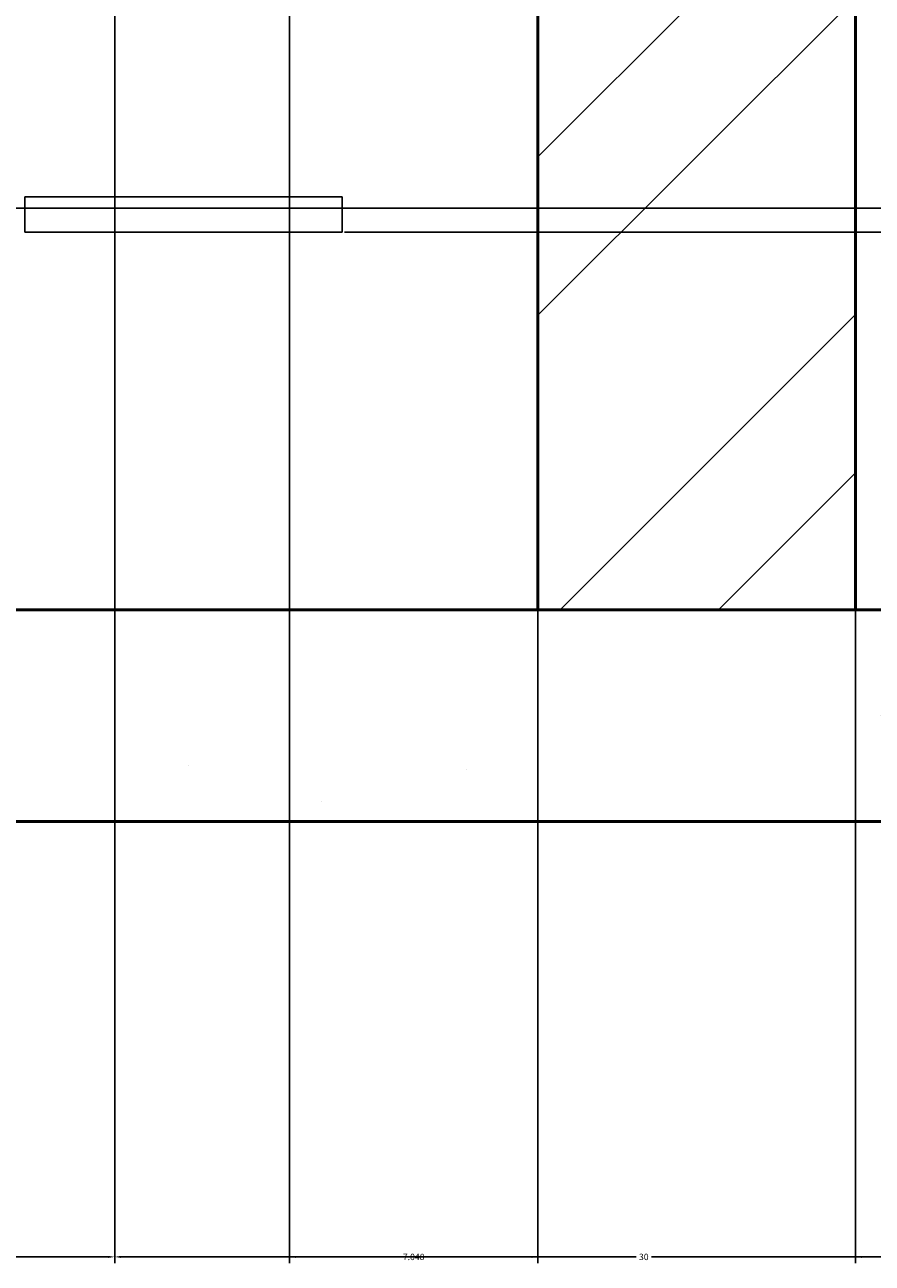
# Model space of a CAD drawing. Units: inches. Extents: x 2812 to 3051, y 1398 to 1659.
# Tile 33 of 65: x 3004 to 3028, y 1398 to 1433. Entities that reach past the tile are written whole.
import ezdxf

# ---------------------------------------------------------------- set-up
doc = ezdxf.new("R2010")
doc.units = ezdxf.units.IN
for name, color, linetype, lineweight in [('A-ANNO-DIMS', 2, 'Continuous', 18), ('S-CONC', 7, 'Continuous', 50), ('S-CONC-PATT', 8, 'Continuous', 18), ('S-STEP', 3, 'Continuous', 25)]:
    doc.layers.add(name, color=color, linetype=linetype, lineweight=lineweight)
doc.styles.get("Standard").update_dxf_attribs({"font": 'arial.ttf'})
doc.dimstyles.get("Standard").update_dxf_attribs({"dimtxt": 0.18, "dimasz": 0.18, "dimexe": 0.18, "dimexo": 0.0625, "dimgap": 0.09, "dimtad": 0, "dimtih": 1, "dimtoh": 1, "dimdec": 4, "dimzin": 0, "dimdsep": 46, "dimtxsty": 'Standard', "dimcen": 0.09, "dimadec": 0, "dimazin": 0, "dimtfac": 1, "dimtdec": 4, "dimtofl": 0, "dimtmove": 0, "dimatfit": 3, "dimfxl": 1, "dimtolj": 1, "dimtzin": 0, "dimarcsym": 0})

# ---------------------------------------------------------------- blocks, each defined once
blk = doc.blocks.new('STEP-IRON-3')
for p, q in [((9, 1), (0, 1)), ((0, 1), (0, 0)), ((9, 0), (9, 1)), ((0, 0), (4.457, 0)), ((0, 0), (9, 0)), ((0, 0), (5.792, 0))]:
    blk.add_line(p, q)
blk = doc.blocks.new('*D33')
at = {"layer": 'A-ANNO-DIMS', "color": 0, "lineweight": -2, "transparency": 16777216}
for p, q in [((3011.337, 1597.982), (3011.337, 1397.505)), ((3018.385, 1559.757), (3018.385, 1397.505)), ((3011.517, 1397.685), (3014.468, 1397.685)), ((3018.205, 1397.685), (3015.254, 1397.685))]:
    blk.add_line(p, q, dxfattribs=at)
at = {"layer": 'A-ANNO-DIMS', "color": 0, "transparency": 16777216}
for points in [[(3011.517, 1397.715), (3011.517, 1397.655), (3011.337, 1397.685)], [(3018.205, 1397.715), (3018.205, 1397.655), (3018.385, 1397.685)]]:
    blk.add_solid(points, dxfattribs=at)
at = {"layer": 'Defpoints', "color": 0, "transparency": 16777216}
for p in [(3011.337, 1598.044), (3018.385, 1559.82), (3018.385, 1397.685)]:
    blk.add_point(p, dxfattribs=at)
at = {"layer": 'A-ANNO-DIMS', "color": 0, "transparency": 16777216, "insert": (3014.861, 1397.685), "char_height": 0.18, "attachment_point": 5}
blk.add_mtext('\\A1;7.048', dxfattribs=at)
blk = doc.blocks.new('*D34')
at = {"layer": 'A-ANNO-DIMS', "color": 0, "lineweight": -2, "transparency": 16777216}
for p, q in [((3038.462, 1593.482), (3038.462, 1397.505)), ((3027.385, 1550.757), (3027.385, 1397.505)), ((3027.565, 1397.685), (3032.468, 1397.685)), ((3038.282, 1397.685), (3033.379, 1397.685))]:
    blk.add_line(p, q, dxfattribs=at)
at = {"layer": 'A-ANNO-DIMS', "color": 0, "transparency": 16777216}
for points in [[(3027.565, 1397.715), (3027.565, 1397.655), (3027.385, 1397.685)], [(3038.282, 1397.715), (3038.282, 1397.655), (3038.462, 1397.685)]]:
    blk.add_solid(points, dxfattribs=at)
at = {"layer": 'Defpoints', "color": 0, "transparency": 16777216}
for p in [(3038.462, 1593.544), (3027.385, 1550.82), (3038.462, 1397.685)]:
    blk.add_point(p, dxfattribs=at)
at = {"layer": 'A-ANNO-DIMS', "color": 0, "transparency": 16777216, "insert": (3032.923, 1397.685), "char_height": 0.18, "attachment_point": 5}
blk.add_mtext('\\A1;11.077', dxfattribs=at)
blk = doc.blocks.new('*D47')
at = {"layer": 'A-ANNO-DIMS', "color": 0, "lineweight": -2, "transparency": 16777216}
for p, q in [((2970.385, 1487.973), (2970.385, 1397.505)), ((3006.385, 1487.973), (3006.385, 1397.505)), ((2970.565, 1397.685), (2988.166, 1397.685)), ((3006.205, 1397.685), (2988.604, 1397.685))]:
    blk.add_line(p, q, dxfattribs=at)
at = {"layer": 'A-ANNO-DIMS', "color": 0, "transparency": 16777216}
for points in [[(2970.565, 1397.715), (2970.565, 1397.655), (2970.385, 1397.685)], [(3006.205, 1397.715), (3006.205, 1397.655), (3006.385, 1397.685)]]:
    blk.add_solid(points, dxfattribs=at)
at = {"layer": 'Defpoints', "color": 0, "transparency": 16777216}
for p in [(2970.385, 1488.035), (3006.385, 1488.035), (3006.385, 1397.685)]:
    blk.add_point(p, dxfattribs=at)
at = {"layer": 'A-ANNO-DIMS', "color": 0, "transparency": 16777216, "insert": (2988.385, 1397.685), "char_height": 0.18, "attachment_point": 5}
blk.add_mtext('\\A1;36', dxfattribs=at)
blk = doc.blocks.new('*D48')
at = {"layer": 'A-ANNO-DIMS', "color": 0, "lineweight": -2, "transparency": 16777216}
for p, q in [((3006.385, 1487.973), (3006.385, 1397.505)), ((3036.385, 1409.973), (3036.385, 1397.505)), ((3006.565, 1397.685), (3021.166, 1397.685)), ((3036.205, 1397.685), (3021.603, 1397.685))]:
    blk.add_line(p, q, dxfattribs=at)
at = {"layer": 'A-ANNO-DIMS', "color": 0, "transparency": 16777216}
for points in [[(3006.565, 1397.715), (3006.565, 1397.655), (3006.385, 1397.685)], [(3036.205, 1397.715), (3036.205, 1397.655), (3036.385, 1397.685)]]:
    blk.add_solid(points, dxfattribs=at)
at = {"layer": 'Defpoints', "color": 0, "transparency": 16777216}
for p in [(3006.385, 1488.035), (3036.385, 1410.035), (3036.385, 1397.685)]:
    blk.add_point(p, dxfattribs=at)
at = {"layer": 'A-ANNO-DIMS', "color": 0, "transparency": 16777216, "insert": (3021.385, 1397.685), "char_height": 0.18, "attachment_point": 5}
blk.add_mtext('\\A1;30', dxfattribs=at)
blk = doc.blocks.new('*D64')
at = {"layer": 'A-ANNO-DIMS', "color": 0, "lineweight": -2, "transparency": 16777216}
for p, q in [((2929.438, 1427.426), (3051.178, 1427.426)), ((3050.998, 1427.246), (3050.998, 1421.913)), ((3050.998, 1416.215), (3050.998, 1421.549)), ((2952.447, 1416.035), (3051.178, 1416.035))]:
    blk.add_line(p, q, dxfattribs=at)
at = {"layer": 'A-ANNO-DIMS', "color": 0, "transparency": 16777216}
for points in [[(3050.968, 1427.246), (3051.028, 1427.246), (3050.998, 1427.426)], [(3050.968, 1416.215), (3051.028, 1416.215), (3050.998, 1416.035)]]:
    blk.add_solid(points, dxfattribs=at)
at = {"layer": 'Defpoints', "color": 0, "transparency": 16777216}
for p in [(2929.375, 1427.426), (3050.998, 1427.426), (2952.385, 1416.035)]:
    blk.add_point(p, dxfattribs=at)
at = {"layer": 'A-ANNO-DIMS', "color": 0, "transparency": 16777216, "insert": (3050.998, 1421.731), "char_height": 0.18, "attachment_point": 5}
blk.add_mtext('\\A1;11.39', dxfattribs=at)
blk = doc.blocks.new('*D65')
at = {"layer": 'A-ANNO-DIMS', "color": 0, "lineweight": -2, "transparency": 16777216}
for p, q in [((2920.62, 1437.426), (3051.178, 1437.426)), ((3050.998, 1437.246), (3050.998, 1432.608)), ((3050.998, 1427.606), (3050.998, 1432.245)), ((2929.438, 1427.426), (3051.178, 1427.426))]:
    blk.add_line(p, q, dxfattribs=at)
at = {"layer": 'A-ANNO-DIMS', "color": 0, "transparency": 16777216}
for points in [[(3050.968, 1437.246), (3051.028, 1437.246), (3050.998, 1437.426)], [(3050.968, 1427.606), (3051.028, 1427.606), (3050.998, 1427.426)]]:
    blk.add_solid(points, dxfattribs=at)
at = {"layer": 'Defpoints', "color": 0, "transparency": 16777216}
for p in [(2920.558, 1437.426), (3050.998, 1437.426), (2929.375, 1427.426)]:
    blk.add_point(p, dxfattribs=at)
at = {"layer": 'A-ANNO-DIMS', "color": 0, "transparency": 16777216, "insert": (3050.998, 1432.426), "char_height": 0.18, "attachment_point": 5}
blk.add_mtext('\\A1;10', dxfattribs=at)
blk = doc.blocks.new('*D78')
at = {"layer": 'A-ANNO-DIMS', "color": 0, "lineweight": -2, "transparency": 16777216}
for p, q in [((3012.899, 1426.747), (3051.178, 1426.747)), ((3050.998, 1426.567), (3050.998, 1421.573)), ((3050.998, 1416.215), (3050.998, 1421.209)), ((3018.447, 1416.035), (3051.178, 1416.035))]:
    blk.add_line(p, q, dxfattribs=at)
at = {"layer": 'A-ANNO-DIMS', "color": 0, "transparency": 16777216}
for points in [[(3050.968, 1426.567), (3051.028, 1426.567), (3050.998, 1426.747)], [(3050.968, 1416.215), (3051.028, 1416.215), (3050.998, 1416.035)]]:
    blk.add_solid(points, dxfattribs=at)
at = {"layer": 'Defpoints', "color": 0, "transparency": 16777216}
for p in [(3012.837, 1426.747), (3050.998, 1426.747), (3018.385, 1416.035)]:
    blk.add_point(p, dxfattribs=at)
at = {"layer": 'A-ANNO-DIMS', "color": 0, "transparency": 16777216, "insert": (3050.998, 1421.391), "char_height": 0.18, "attachment_point": 5}
blk.add_mtext('\\A1;10.712', dxfattribs=at)
blk = doc.blocks.new('*D79')
at = {"layer": 'A-ANNO-DIMS', "color": 0, "lineweight": -2, "transparency": 16777216}
for p, q in [((3003.284, 1436.747), (3051.178, 1436.747)), ((3050.998, 1436.567), (3050.998, 1431.929)), ((3050.998, 1426.927), (3050.998, 1431.565)), ((3012.899, 1426.747), (3051.178, 1426.747))]:
    blk.add_line(p, q, dxfattribs=at)
at = {"layer": 'A-ANNO-DIMS', "color": 0, "transparency": 16777216}
for points in [[(3050.968, 1436.567), (3051.028, 1436.567), (3050.998, 1436.747)], [(3050.968, 1426.927), (3051.028, 1426.927), (3050.998, 1426.747)]]:
    blk.add_solid(points, dxfattribs=at)
at = {"layer": 'Defpoints', "color": 0, "transparency": 16777216}
for p in [(3003.221, 1436.747), (3050.998, 1436.747), (3012.837, 1426.747)]:
    blk.add_point(p, dxfattribs=at)
at = {"layer": 'A-ANNO-DIMS', "color": 0, "transparency": 16777216, "insert": (3050.998, 1431.747), "char_height": 0.18, "attachment_point": 5}
blk.add_mtext('\\A1;10', dxfattribs=at)

msp = doc.modelspace()

# ---------------------------------------------------------------- hatches: boundary and pattern name
at = {"layer": 'S-CONC-PATT'}
h = msp.add_hatch(dxfattribs=at)
h.set_pattern_fill('ANSI32', color=256)
h.paths.add_polyline_path([(3027.3849, 1646.82), (2835.3849, 1646.82), (2835.3849, 1603.2296), (2844.3849, 1603.2296), (2844.3849, 1637.82), (3018.3849, 1637.82), (3018.3849, 1602.5441), (3027.3849, 1602.5441)])
h.paths.add_polyline_path([(2844.3849, 1594.2296), (2835.3849, 1594.2296), (2835.3849, 1550.82), (3027.3849, 1550.82), (3027.3849, 1593.5441), (3018.3849, 1593.5441), (3018.3849, 1559.82), (2844.3849, 1559.82)])
h.paths.add_polyline_path([(2844.3849, 1482.0354), (2835.3849, 1482.0354), (2835.3849, 1463.4959), (2844.3849, 1463.4959)])
h.paths.add_polyline_path([(2844.3849, 1461.4959), (2835.3849, 1461.4959), (2835.3849, 1416.0354), (2844.3849, 1416.0354)])
h.paths.add_polyline_path([(3027.3849, 1482.0354), (3018.3849, 1482.0354), (3018.3849, 1463.2854), (3027.3849, 1463.2854)])
h.paths.add_polyline_path([(3027.3849, 1461.2854), (3018.3849, 1461.2854), (3018.3849, 1416.0354), (3027.3849, 1416.0354)])
h.paths.add_polyline_path([(2961.3849, 1448.4738), (2952.3849, 1448.4738), (2952.3849, 1416.0354), (2961.3849, 1416.0354)])
h.paths.add_polyline_path([(2961.3849, 1462.3026), (2952.3849, 1462.3026), (2952.3849, 1450.4738), (2961.3849, 1450.4738)])
h.paths.add_polyline_path([(2961.3849, 1472.0354), (2952.3849, 1472.0354), (2952.3849, 1462.3026), (2961.3849, 1462.3026)])
h = msp.add_hatch(dxfattribs=at)
h.set_pattern_fill('AR-SAND', color=256, scale=0.3)
h.paths.add_polyline_path([(3036.3849, 1416.0354), (3027.3849, 1416.0354), (2826.3849, 1416.0354), (2826.3849, 1410.0354), (2835.3849, 1410.0354), (3036.3849, 1410.0354)])
h.paths.add_polyline_path([(2970.3849, 1488.0354), (2969.3849, 1488.0354), (2941.3849, 1488.0354), (2941.3849, 1482.0354), (2970.3849, 1482.0354)])
h.paths.add_polyline_path([(3036.3849, 1488.0354), (3035.3849, 1488.0354), (3006.3849, 1488.0354), (3006.3849, 1482.0354), (3027.3849, 1482.0354), (3036.3849, 1482.0354)])
h.paths.add_polyline_path([(3034.3849, 1490.0354), (3008.3849, 1490.0354), (3008.3849, 1489.0354), (3034.3849, 1489.0354)])
h.paths.add_polyline_path([(3035.3849, 1489.0354), (3034.3849, 1489.0354), (3007.3849, 1489.0354), (3007.3849, 1488.0354), (3035.3849, 1488.0354)])
h.paths.add_polyline_path([(2968.3849, 1490.0354), (2943.3849, 1490.0354), (2943.3849, 1489.0354), (2968.3849, 1489.0354)])
h.paths.add_polyline_path([(2969.3849, 1489.0354), (2968.3849, 1489.0354), (2942.3849, 1489.0354), (2942.3849, 1488.0354), (2969.3849, 1488.0354)])
h.paths.add_polyline_path([(2896.3849, 1488.0354), (2826.3849, 1488.0354), (2826.3849, 1482.0354), (2896.3849, 1482.0354)])
h.paths.add_polyline_path([(2895.3849, 1489.0354), (2894.3849, 1489.0354), (2827.3849, 1489.0354), (2827.3849, 1488.0354), (2895.3849, 1488.0354)])
h.paths.add_polyline_path([(2894.3849, 1490.0354), (2828.3849, 1490.0354), (2828.3849, 1489.0354), (2894.3849, 1489.0354)])
h = msp.add_hatch(dxfattribs=at)
h.set_pattern_fill('AR-CONC', color=256, scale=0.3)
h.paths.add_polyline_path([(3036.3849, 1416.0354), (3027.3849, 1416.0354), (2826.3849, 1416.0354), (2826.3849, 1410.0354), (2835.3849, 1410.0354), (3036.3849, 1410.0354)])

# ---------------------------------------------------------------- linework, layer by layer
at = {"layer": 'S-CONC'}
for p, q in [((3018.3849, 1482.0354), (3018.3849, 1416.0354)), ((3027.3849, 1482.0354), (3027.3849, 1416.0354)), ((2826.3849, 1416.0354), (3027.3849, 1416.0354)), ((3027.3849, 1416.0354), (3036.3849, 1416.0354)), ((2835.3849, 1410.0354), (3036.3849, 1410.0354))]:
    msp.add_line(p, q, dxfattribs=at)

# ---------------------------------------------------------------- block references
at = {"layer": 'S-STEP'}
msp.add_blockref('STEP-IRON-3', (3003.837, 1426.747), dxfattribs=at)

# ---------------------------------------------------------------- dimensions: what is measured, and where the dimension line sits
at = {"layer": 'A-ANNO-DIMS'}
for base, p1, p2, override, picture, middle in [((3018.3849, 1397.6854), (3011.3373, 1598.0441), (3018.3849, 1559.82), {"dimdec": 3, "dimlfac": 1, "dimrnd": 0, "dimzin": 0, "dimdsep": 46, "dimlunit": 2}, '*D33', (3014.8611, 1397.6854)), ((3038.4621, 1397.6854), (3027.3849, 1550.82), (3038.4621, 1593.5441), {"dimdec": 3, "dimlfac": 1, "dimrnd": 0, "dimzin": 0, "dimdsep": 46, "dimlunit": 2}, '*D34', (3032.9235, 1397.6854)), ((3006.3849, 1397.6854), (2970.3849, 1488.0354), (3006.3849, 1488.0354), {"dimdec": 0, "dimlfac": 1, "dimrnd": 0, "dimzin": 0, "dimdsep": 46, "dimlunit": 2}, '*D47', (2988.3849, 1397.6854)), ((3036.3849, 1397.6854), (3006.3849, 1488.0354), (3036.3849, 1410.0354), {"dimdec": 0, "dimlfac": 1, "dimrnd": 0, "dimzin": 0, "dimdsep": 46, "dimlunit": 2}, '*D48', (3021.3849, 1397.6854))]:
    dim = msp.add_linear_dim(base=base, p1=p1, p2=p2, dimstyle='Standard', override=override, dxfattribs=at)
    dim.commit()
    dim.dimension.update_dxf_attribs({"geometry": picture, "text_midpoint": middle})
for base, p1, p2, override, picture, middle in [((3050.998, 1437.4265), (2929.3751, 1427.4265), (2920.5577, 1437.4265), {"dimdec": 0, "dimlfac": 1, "dimrnd": 0, "dimzin": 0, "dimdsep": 46, "dimlunit": 2}, '*D65', (3050.998, 1432.4265)), ((3050.998, 1436.7474), (3012.8368, 1426.7474), (3003.2213, 1436.7474), {"dimdec": 0, "dimlfac": 1, "dimrnd": 0, "dimzin": 0, "dimdsep": 46, "dimlunit": 2}, '*D79', (3050.998, 1431.7474)), ((3050.998, 1427.4265), (2952.3849, 1416.0354), (2929.3751, 1427.4265), {"dimdec": 2, "dimlfac": 1, "dimrnd": 0, "dimzin": 0, "dimdsep": 46, "dimlunit": 2}, '*D64', (3050.998, 1421.7309)), ((3050.998, 1426.7474), (3018.3849, 1416.0354), (3012.8368, 1426.7474), {"dimdec": 3, "dimlfac": 1, "dimrnd": 0, "dimzin": 0, "dimdsep": 46, "dimlunit": 2}, '*D78', (3050.998, 1421.3914))]:
    dim = msp.add_linear_dim(base=base, p1=p1, p2=p2, angle=90, dimstyle='Standard', override=override, dxfattribs=at)
    dim.commit()
    dim.dimension.update_dxf_attribs({"geometry": picture, "text_midpoint": middle})

doc.saveas('drawing.dxf')
